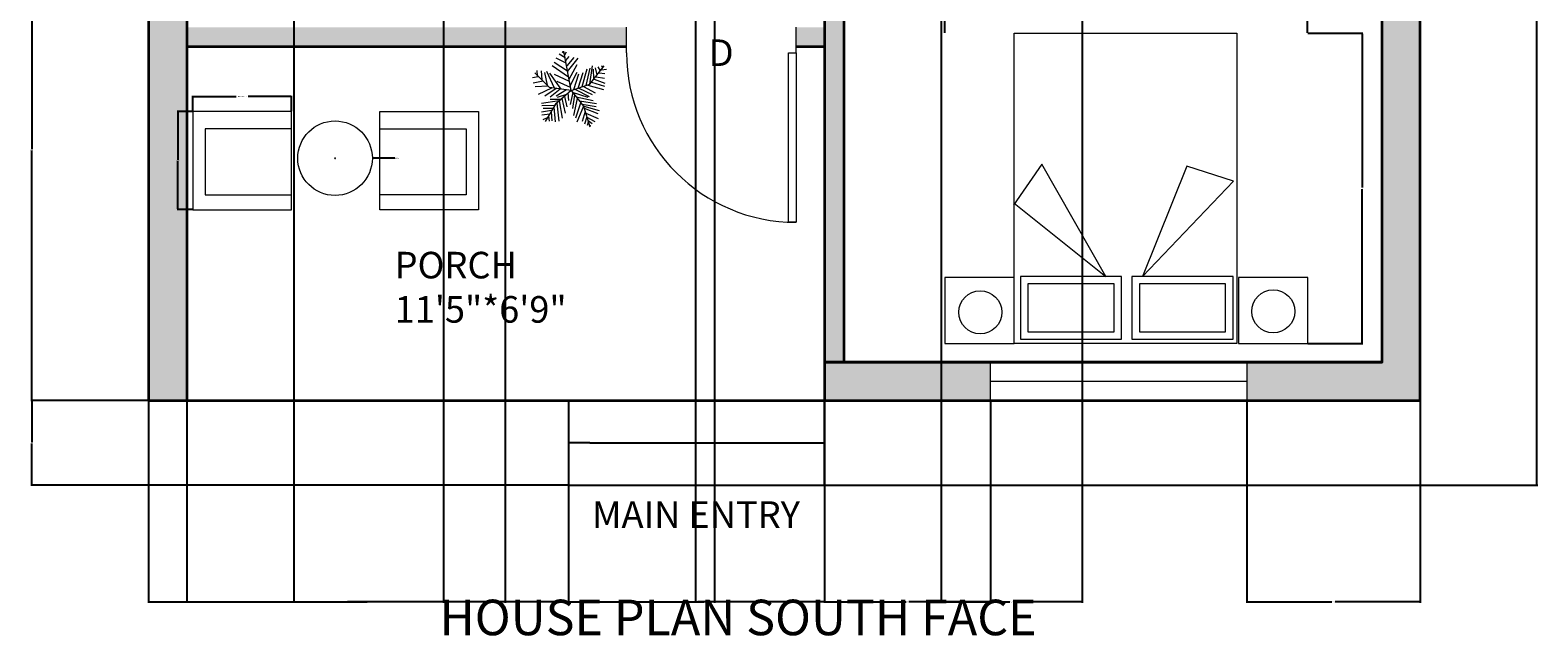
# Model space of a CAD drawing. Units: inches. Extents: x 1841 to 2210, y 2173 to 2736.
# Tile 1 of 4: x 1841 to 2197, y 2173 to 2316. Entities that reach past the tile are written whole.
import ezdxf

# ---------------------------------------------------------------- set-up
doc = ezdxf.new("R2010")
doc.units = ezdxf.units.IN
for name, color, linetype, lineweight in [('A-ANNO-DIMS', 2, 'Continuous', 18), ('A-AREA-IDEN', 10, 'Continuous', 18), ('A-FLOR-STRS', 7, 'Continuous', 25), ('A-FURN', 8, 'Continuous', 18), ('A-WALL', 7, 'Continuous', 35), ('A-WALL-PATT', 252, 'Continuous', 13), ('BED', 120, 'Continuous', 18), ('DOOR', 50, 'Continuous', 18), ('TEXT', 10, 'Continuous', 18), ('TREE', 70, 'Continuous', 13), ('WIN', 193, 'Continuous', 18)]:
    doc.layers.add(name, color=color, linetype=linetype, lineweight=lineweight)
doc.styles.get("Standard").update_dxf_attribs({"font": 'arial.ttf'})
doc.dimstyles.get("Standard").update_dxf_attribs({"dimtxt": 0.18, "dimasz": 0.18, "dimexe": 0.18, "dimexo": 0.0625, "dimgap": 0.09, "dimtad": 0, "dimtih": 1, "dimtoh": 1, "dimdec": 4, "dimzin": 0, "dimdsep": 46, "dimtxsty": 'Standard', "dimcen": 0.09, "dimadec": 0, "dimazin": 0, "dimtfac": 1, "dimtdec": 4, "dimtofl": 0, "dimtmove": 0, "dimatfit": 3, "dimfxl": 1, "dimtolj": 1, "dimtzin": 0, "dimarcsym": 0})

# ---------------------------------------------------------------- blocks, each defined once
blk = doc.blocks.new('*U2')
for p, q in [((0, 0), (0, -6)), ((40, 0), (40, -6))]:
    blk.add_line(p, q)
blk.add_lwpolyline([(0, 0), (0, 40), (1.75, 40), (1.75, 0)], close=True)
blk.add_arc((0, 0), 40, 0, 90)
blk = doc.blocks.new('*U6')
for p, q in [((-7.288, 39.707), (-21.778, 46.673)), ((-8.737, 47.138), (-17.069, 52.711)), ((-10.186, 53.64), (-13.084, 55.962)), ((0, 0), (-10.5, 57)), ((-9.099, 51.782), (-6.563, 55.962)), ((-7.65, 43.423), (-2.578, 49.46)), ((-5.839, 35.992), (4.667, 48.067)), ((-5.114, 27.632), (10.463, 46.673)), ((-31.5, 4.5), (-52.5, 25.5)), ((-48.585, 21.131), (-49.309, 29.026)), ((-43.513, 28.561), (-42.427, 15.558)), ((-38.442, 26.239), (-34.819, 7.663)), ((-35.544, 28.097), (-24.314, 3.947)), ((-14.533, 2.09), (-30.834, 25.31)), ((-3.665, 19.273), (-27.574, 35.527)), ((-5.114, 28.097), (-24.676, 40.636)), ((-24.314, 23.917), (-2.941, 13.7)), ((-2.941, 16.486), (8.652, 37.85)), ((-1.129, 6.734), (9.014, 26.704)), ((3.942, 1.625), (11.187, 24.381)), ((10.101, 3.483), (17.708, 26.239)), ((16.259, 5.805), (23.142, 31.348)), ((22.055, 7.198), (27.489, 32.277)), ((27, 9), (48, 36)), ((27.127, 9.056), (31.112, 35.992)), ((31.836, 30.883), (32.561, 16.486)), ((35.096, 32.741), (37.27, 22.524)), ((38.719, 34.134), (41.979, 28.561)), ((40.53, 25.775), (48.862, 24.846)), ((43.791, 29.954), (51.036, 30.883)), ((44.153, 36.456), (45.239, 32.741)), ((-47.498, 19.737), (-55.83, 18.344)), ((-40.615, 13.7), (-55.105, 10.913)), ((-33.37, 6.269), (-52.207, 5.34)), ((-28.299, 3.483), (-47.86, -5.805)), ((-21.416, 3.018), (-38.079, -8.128)), ((0, 0), (-31.5, 4.5)), ((-15.982, 2.09), (-30.11, -9.521)), ((0, 0), (-22.5, -19.5)), ((-6.563, 1.161), (-21.416, -8.128)), ((-20.691, 13.7), (-1.129, 4.876)), ((0, 0), (27, 9)), ((0, 0), (18, -22.5)), ((6.478, 1.625), (26.04, -8.592)), ((11.187, 3.483), (30.749, -5.805)), ((18.07, 5.805), (35.096, -3.483)), ((24.229, 7.663), (46.688, 1.625)), ((29.662, 12.307), (48.137, 6.269)), ((33.285, 16.486), (48.862, 10.913)), ((36.183, 19.737), (48.137, 17.88)), ((-17.431, -15.094), (-42.789, -18.809)), ((-24.314, -21.596), (-42.427, -22.06)), ((-22.5, -19.5), (-37.5, -45)), ((-15.257, -12.772), (-30.11, -12.772)), ((-20.691, -18.345), (-17.793, -44.352)), ((-6.563, -5.805), (-19.967, -9.985)), ((-17.069, -15.094), (-12.721, -40.172)), ((-13.446, -11.378), (-8.737, -32.741)), ((-9.461, -8.592), (-6.201, -23.453)), ((-4.752, -3.483), (-3.665, -14.629)), ((2.493, -3.019), (-1.491, -20.202)), ((1.769, -2.555), (24.229, -9.521)), ((5.029, -6.27), (2.131, -25.775)), ((9.014, -11.378), (3.58, -35.992)), ((14.085, -16.951), (6.478, -40.172)), ((7.565, -9.056), (32.198, -14.629)), ((12.274, -15.094), (36.907, -18.809)), ((16.259, -19.738), (36.183, -22.989)), ((-28.299, -29.026), (-42.789, -31.348)), ((-30.834, -34.135), (-42.427, -35.528)), ((-34.457, -39.708), (-40.978, -42.494)), ((-26.849, -26.24), (-40.253, -25.775)), ((-32.646, -36.921), (-31.921, -44.352)), ((-29.023, -30.884), (-27.936, -43.887)), ((-25.038, -23.918), (-22.865, -45.281)), ((18.07, -22.524), (8.289, -45.745)), ((20.244, -30.419), (15.897, -44.816)), ((18, -22.5), (27, -52.5)), ((18.433, -22.524), (40.53, -29.026)), ((19.157, -25.311), (38.719, -33.206)), ((22.78, -37.85), (19.519, -48.532)), ((21.331, -32.741), (39.081, -40.636)), ((22.78, -38.314), (34.372, -44.816)), ((24.591, -43.423), (30.749, -47.603)), ((24.591, -45.745), (23.142, -50.854)), ((26.764, -49.925), (28.213, -50.854))]:
    blk.add_line(p, q)
blk = doc.blocks.new('BED-DOUBLE-WITH-NIGHTSTANDS')
for p, q in [((33.07, 69.27), (15.79, 47.62)), ((42.3, 62.7), (32.63, 69.37)), ((15.79, 47.62), (42.3, 62.7)), ((15.79, 39), (38.26, 17.46)), ((41.84, 28.47), (15.79, 39)), ((38.26, 17.46), (41.84, 28.47))]:
    blk.add_line(p, q)
for points in [[(0, 69.27), (15.55, 69.27), (15.55, 85.57), (0, 85.57)], [(0, 69.27), (73.23, 69.27), (73.23, 16.72), (0, 16.72)], [(1.03, 43.89), (15.79, 43.89), (15.79, 67.76), (1.03, 67.76)], [(2.79, 45.65), (14.04, 45.65), (14.04, 66), (2.79, 66)], [(1.03, 17.59), (15.79, 17.59), (15.79, 41.47), (1.03, 41.47)], [(2.79, 19.35), (14.04, 19.35), (14.04, 39.71), (2.79, 39.71)], [(0, 0), (15.55, 0), (15.55, 16.3), (0, 16.3)]]:
    blk.add_lwpolyline(points, close=True)
for centre in [(7.36, 77.24), (7.58, 8.12)]:
    blk.add_circle(centre, 5.08)
blk = doc.blocks.new('WIN-60IN-NOM')
blk.add_line((4.5, 0), (4.5, 60.52))
blk.add_lwpolyline([(0, 60.52), (9, 60.52), (9, 0), (0, 0)], close=True)
blk = doc.blocks.new('CHAIR-PORCH')
for p, q in [((23.32, 23.17), (0, 23.17)), ((0, 23.17), (0, 0)), ((23.32, 19.05), (23.32, 23.17)), ((23.32, 0), (23.32, 11.27)), ((0, 0), (23.32, 0))]:
    blk.add_line(p, q)
blk.add_lwpolyline([(23.32, 19.05), (2.95, 19.05), (2.95, 3.5), (23.32, 3.5)], close=True)
blk = doc.blocks.new('*D16')
at = {"layer": 'A-ANNO-DIMS', "color": 0, "lineweight": -2, "transparency": 16777216}
for p, q in [((2056.93, 2315.11), (2056.93, 2328.07)), ((2057.11, 2327.89), (2098.62, 2327.89)), ((2142.32, 2327.89), (2100.81, 2327.89)), ((2142.5, 2315.11), (2142.5, 2328.07))]:
    blk.add_line(p, q, dxfattribs=at)
at = {"layer": 'A-ANNO-DIMS', "color": 0, "transparency": 16777216}
for points in [[(2057.11, 2327.92), (2057.11, 2327.86), (2056.93, 2327.89)], [(2142.32, 2327.92), (2142.32, 2327.86), (2142.5, 2327.89)]]:
    blk.add_solid(points, dxfattribs=at)
at = {"layer": 'Defpoints', "color": 0, "transparency": 16777216}
for p in [(2056.93, 2327.89), (2056.93, 2315.05), (2142.5, 2315.05)]:
    blk.add_point(p, dxfattribs=at)
at = {"layer": 'A-ANNO-DIMS', "color": 0, "transparency": 16777216, "insert": (2099.72, 2327.89), "char_height": 0.18, "attachment_point": 5}
blk.add_mtext('\\A1;BED SET 86 TYP.', dxfattribs=at)
blk = doc.blocks.new('*D17')
at = {"layer": 'A-ANNO-DIMS', "color": 0, "lineweight": -2, "transparency": 16777216}
for p, q in [((2142.57, 2315.05), (2155.52, 2315.05)), ((2155.34, 2314.87), (2155.34, 2278.62)), ((2155.34, 2242), (2155.34, 2278.25)), ((2142.57, 2241.82), (2155.52, 2241.82))]:
    blk.add_line(p, q, dxfattribs=at)
at = {"layer": 'A-ANNO-DIMS', "color": 0, "transparency": 16777216}
for points in [[(2155.31, 2314.87), (2155.37, 2314.87), (2155.34, 2315.05)], [(2155.31, 2242), (2155.37, 2242), (2155.34, 2241.82)]]:
    blk.add_solid(points, dxfattribs=at)
at = {"layer": 'Defpoints', "color": 0, "transparency": 16777216}
for p in [(2142.5, 2315.05), (2155.34, 2315.05), (2142.5, 2241.82)]:
    blk.add_point(p, dxfattribs=at)
at = {"layer": 'A-ANNO-DIMS', "color": 0, "transparency": 16777216, "insert": (2155.34, 2278.44), "char_height": 0.18, "attachment_point": 5}
blk.add_mtext('\\A1;73 TYP.', dxfattribs=at)
blk = doc.blocks.new('*D18')
at = {"layer": 'A-ANNO-DIMS', "color": 0, "lineweight": -2, "transparency": 16777216}
for p, q in [((1879.48, 2296.62), (1879.48, 2300.23)), ((1879.66, 2300.05), (1889.7, 2300.05)), ((1902.62, 2300.05), (1892.58, 2300.05)), ((1902.8, 2296.62), (1902.8, 2300.23))]:
    blk.add_line(p, q, dxfattribs=at)
at = {"layer": 'A-ANNO-DIMS', "color": 0, "transparency": 16777216}
for points in [[(1879.66, 2300.08), (1879.66, 2300.02), (1879.48, 2300.05)], [(1902.62, 2300.08), (1902.62, 2300.02), (1902.8, 2300.05)]]:
    blk.add_solid(points, dxfattribs=at)
at = {"layer": 'Defpoints', "color": 0, "transparency": 16777216}
for p in [(1902.8, 2300.05), (1879.48, 2296.55), (1902.8, 2296.55)]:
    blk.add_point(p, dxfattribs=at)
at = {"layer": 'A-ANNO-DIMS', "color": 0, "transparency": 16777216, "insert": (1891.14, 2300.05), "char_height": 0.18, "attachment_point": 5}
blk.add_mtext('\\A1;PORCH CHAIR 23 TYP.', dxfattribs=at)
blk = doc.blocks.new('*D19')
at = {"layer": 'A-ANNO-DIMS', "color": 0, "lineweight": -2, "transparency": 16777216}
for p, q in [((1879.42, 2296.55), (1875.8, 2296.55)), ((1875.98, 2296.37), (1875.98, 2285.15)), ((1875.98, 2273.57), (1875.98, 2284.79)), ((1879.42, 2273.39), (1875.8, 2273.39))]:
    blk.add_line(p, q, dxfattribs=at)
at = {"layer": 'A-ANNO-DIMS', "color": 0, "transparency": 16777216}
for points in [[(1875.95, 2296.37), (1876.01, 2296.37), (1875.98, 2296.55)], [(1875.95, 2273.57), (1876.01, 2273.57), (1875.98, 2273.39)]]:
    blk.add_solid(points, dxfattribs=at)
at = {"layer": 'Defpoints', "color": 0, "transparency": 16777216}
for p in [(1875.98, 2296.55), (1879.48, 2296.55), (1879.48, 2273.39)]:
    blk.add_point(p, dxfattribs=at)
at = {"layer": 'A-ANNO-DIMS', "color": 0, "transparency": 16777216, "insert": (1875.98, 2284.97), "char_height": 0.18, "attachment_point": 5}
blk.add_mtext('\\A1;23 TYP.', dxfattribs=at)
blk = doc.blocks.new('*D23')
at = {"layer": 'A-ANNO-DIMS', "color": 0, "lineweight": -2, "transparency": 16777216}
for p, q in [((2169.11, 2708.41), (2196.78, 2708.41)), ((2196.6, 2708.23), (2196.6, 2458.59)), ((2196.6, 2208.59), (2196.6, 2458.22)), ((2028.61, 2208.41), (2196.78, 2208.41))]:
    blk.add_line(p, q, dxfattribs=at)
at = {"layer": 'A-ANNO-DIMS', "color": 0, "transparency": 16777216}
for points in [[(2196.57, 2708.23), (2196.63, 2708.23), (2196.6, 2708.41)], [(2196.57, 2208.59), (2196.63, 2208.59), (2196.6, 2208.41)]]:
    blk.add_solid(points, dxfattribs=at)
at = {"layer": 'Defpoints', "color": 0, "transparency": 16777216}
for p in [(2169.05, 2708.41), (2196.6, 2708.41), (2028.55, 2208.41)]:
    blk.add_point(p, dxfattribs=at)
at = {"layer": 'A-ANNO-DIMS', "color": 0, "transparency": 16777216, "insert": (2196.6, 2458.41), "char_height": 0.18, "attachment_point": 5}
blk.add_mtext('\\A1;500', dxfattribs=at)
blk = doc.blocks.new('*D24')
at = {"layer": 'A-ANNO-DIMS', "color": 0, "lineweight": -2, "transparency": 16777216}
for p, q in [((1968.08, 2228.41), (1841.32, 2228.41)), ((1841.5, 2228.23), (1841.5, 2218.59)), ((1841.5, 2208.59), (1841.5, 2218.22)), ((1968.08, 2208.41), (1841.32, 2208.41))]:
    blk.add_line(p, q, dxfattribs=at)
at = {"layer": 'A-ANNO-DIMS', "color": 0, "transparency": 16777216}
for points in [[(1841.47, 2228.23), (1841.53, 2228.23), (1841.5, 2228.41)], [(1841.47, 2208.59), (1841.53, 2208.59), (1841.5, 2208.41)]]:
    blk.add_solid(points, dxfattribs=at)
at = {"layer": 'Defpoints', "color": 0, "transparency": 16777216}
for p in [(1841.5, 2228.41), (1968.15, 2228.41), (1968.15, 2208.41)]:
    blk.add_point(p, dxfattribs=at)
at = {"layer": 'A-ANNO-DIMS', "color": 0, "transparency": 16777216, "insert": (1841.5, 2218.41), "char_height": 0.18, "attachment_point": 5}
blk.add_mtext('\\A1;20', dxfattribs=at)
blk = doc.blocks.new('*D25')
at = {"layer": 'A-ANNO-DIMS', "color": 0, "lineweight": -2, "transparency": 16777216}
for p, q in [((1869.05, 2228.34), (1869.05, 2180.68)), ((1968.15, 2228.34), (1968.15, 2180.68)), ((1869.23, 2180.86), (1918.29, 2180.86)), ((1967.97, 2180.86), (1918.9, 2180.86))]:
    blk.add_line(p, q, dxfattribs=at)
at = {"layer": 'A-ANNO-DIMS', "color": 0, "transparency": 16777216}
for points in [[(1869.23, 2180.89), (1869.23, 2180.83), (1869.05, 2180.86)], [(1967.97, 2180.89), (1967.97, 2180.83), (1968.15, 2180.86)]]:
    blk.add_solid(points, dxfattribs=at)
at = {"layer": 'Defpoints', "color": 0, "transparency": 16777216}
for p in [(1869.05, 2228.41), (1968.15, 2228.41), (1968.15, 2180.86)]:
    blk.add_point(p, dxfattribs=at)
at = {"layer": 'A-ANNO-DIMS', "color": 0, "transparency": 16777216, "insert": (1918.6, 2180.86), "char_height": 0.18, "attachment_point": 5}
blk.add_mtext('\\A1;99.1', dxfattribs=at)
blk = doc.blocks.new('*D26')
at = {"layer": 'A-ANNO-DIMS', "color": 0, "lineweight": -2, "transparency": 16777216}
for p, q in [((1968.15, 2208.34), (1968.15, 2180.68)), ((2028.55, 2208.34), (2028.55, 2180.68)), ((1968.33, 2180.86), (1998.02, 2180.86)), ((2028.37, 2180.86), (1998.67, 2180.86))]:
    blk.add_line(p, q, dxfattribs=at)
at = {"layer": 'A-ANNO-DIMS', "color": 0, "transparency": 16777216}
for points in [[(1968.33, 2180.89), (1968.33, 2180.83), (1968.15, 2180.86)], [(2028.37, 2180.89), (2028.37, 2180.83), (2028.55, 2180.86)]]:
    blk.add_solid(points, dxfattribs=at)
at = {"layer": 'Defpoints', "color": 0, "transparency": 16777216}
for p in [(1968.15, 2208.41), (2028.55, 2208.41), (2028.55, 2180.86)]:
    blk.add_point(p, dxfattribs=at)
at = {"layer": 'A-ANNO-DIMS', "color": 0, "transparency": 16777216, "insert": (1998.35, 2180.86), "char_height": 0.18, "attachment_point": 5}
blk.add_mtext('\\A1;60.4', dxfattribs=at)
blk = doc.blocks.new('*D27')
at = {"layer": 'A-ANNO-DIMS', "color": 0, "lineweight": -2, "transparency": 16777216}
for p, q in [((2028.55, 2228.34), (2028.55, 2180.68)), ((2067.65, 2228.34), (2067.65, 2180.68)), ((2028.73, 2180.86), (2047.8, 2180.86)), ((2067.47, 2180.86), (2048.41, 2180.86))]:
    blk.add_line(p, q, dxfattribs=at)
at = {"layer": 'A-ANNO-DIMS', "color": 0, "transparency": 16777216}
for points in [[(2028.73, 2180.89), (2028.73, 2180.83), (2028.55, 2180.86)], [(2067.47, 2180.89), (2067.47, 2180.83), (2067.65, 2180.86)]]:
    blk.add_solid(points, dxfattribs=at)
at = {"layer": 'Defpoints', "color": 0, "transparency": 16777216}
for p in [(2028.55, 2228.41), (2067.65, 2228.41), (2067.65, 2180.86)]:
    blk.add_point(p, dxfattribs=at)
at = {"layer": 'A-ANNO-DIMS', "color": 0, "transparency": 16777216, "insert": (2048.1, 2180.86), "char_height": 0.18, "attachment_point": 5}
blk.add_mtext('\\A1;39.1', dxfattribs=at)
blk = doc.blocks.new('*D28')
at = {"layer": 'A-ANNO-DIMS', "color": 0, "lineweight": -2, "transparency": 16777216}
for p, q in [((2128.17, 2228.34), (2128.17, 2180.68)), ((2169.05, 2228.34), (2169.05, 2180.68)), ((2128.35, 2180.86), (2148.21, 2180.86)), ((2168.87, 2180.86), (2149.01, 2180.86))]:
    blk.add_line(p, q, dxfattribs=at)
at = {"layer": 'A-ANNO-DIMS', "color": 0, "transparency": 16777216}
for points in [[(2128.35, 2180.89), (2128.35, 2180.83), (2128.17, 2180.86)], [(2168.87, 2180.89), (2168.87, 2180.83), (2169.05, 2180.86)]]:
    blk.add_solid(points, dxfattribs=at)
at = {"layer": 'Defpoints', "color": 0, "transparency": 16777216}
for p in [(2128.17, 2228.41), (2169.05, 2228.41), (2128.17, 2180.86)]:
    blk.add_point(p, dxfattribs=at)
at = {"layer": 'A-ANNO-DIMS', "color": 0, "transparency": 16777216, "insert": (2148.61, 2180.86), "char_height": 0.18, "attachment_point": 5}
blk.add_mtext('\\A1;40.88', dxfattribs=at)
blk = doc.blocks.new('*D29')
at = {"layer": 'A-ANNO-DIMS', "color": 0, "lineweight": -2, "transparency": 16777216}
for p, q in [((1868.99, 2346.57), (1841.32, 2346.57)), ((1841.5, 2346.39), (1841.5, 2287.67)), ((1841.5, 2228.59), (1841.5, 2287.31)), ((1868.99, 2228.41), (1841.32, 2228.41))]:
    blk.add_line(p, q, dxfattribs=at)
at = {"layer": 'A-ANNO-DIMS', "color": 0, "transparency": 16777216}
for points in [[(1841.47, 2346.39), (1841.53, 2346.39), (1841.5, 2346.57)], [(1841.47, 2228.59), (1841.53, 2228.59), (1841.5, 2228.41)]]:
    blk.add_solid(points, dxfattribs=at)
at = {"layer": 'Defpoints', "color": 0, "transparency": 16777216}
for p in [(1841.5, 2346.57), (1869.05, 2346.57), (1869.05, 2228.41)]:
    blk.add_point(p, dxfattribs=at)
at = {"layer": 'A-ANNO-DIMS', "color": 0, "transparency": 16777216, "insert": (1841.5, 2287.49), "char_height": 0.18, "attachment_point": 5}
blk.add_mtext('\\A1;118.17', dxfattribs=at)
blk = doc.blocks.new('*D40')
at = {"layer": 'A-ANNO-DIMS', "color": 0, "lineweight": -2, "transparency": 16777216}
for p, q in [((1903.36, 2465.22), (1903.36, 2180.68)), ((1938.67, 2465.22), (1938.67, 2180.68)), ((1903.54, 2180.86), (1920.64, 2180.86)), ((1938.49, 2180.86), (1921.39, 2180.86))]:
    blk.add_line(p, q, dxfattribs=at)
at = {"layer": 'A-ANNO-DIMS', "color": 0, "transparency": 16777216}
for points in [[(1903.54, 2180.89), (1903.54, 2180.83), (1903.36, 2180.86)], [(1938.49, 2180.89), (1938.49, 2180.83), (1938.67, 2180.86)]]:
    blk.add_solid(points, dxfattribs=at)
at = {"layer": 'Defpoints', "color": 0, "transparency": 16777216}
for p in [(1903.36, 2465.28), (1938.67, 2465.28), (1938.67, 2180.86)]:
    blk.add_point(p, dxfattribs=at)
at = {"layer": 'A-ANNO-DIMS', "color": 0, "transparency": 16777216, "insert": (1921.01, 2180.86), "char_height": 0.18, "attachment_point": 5}
blk.add_mtext('\\A1;35.31', dxfattribs=at)
blk = doc.blocks.new('*D42')
at = {"layer": 'A-ANNO-DIMS', "color": 0, "lineweight": -2, "transparency": 16777216}
for p, q in [((1878.05, 2550.84), (1878.05, 2180.68)), ((1953.17, 2550.84), (1953.17, 2180.68)), ((1878.23, 2180.86), (1915.22, 2180.86)), ((1952.99, 2180.86), (1916, 2180.86))]:
    blk.add_line(p, q, dxfattribs=at)
at = {"layer": 'A-ANNO-DIMS', "color": 0, "transparency": 16777216}
for points in [[(1878.23, 2180.89), (1878.23, 2180.83), (1878.05, 2180.86)], [(1952.99, 2180.89), (1952.99, 2180.83), (1953.17, 2180.86)]]:
    blk.add_solid(points, dxfattribs=at)
at = {"layer": 'Defpoints', "color": 0, "transparency": 16777216}
for p in [(1878.05, 2550.91), (1953.17, 2550.91), (1953.17, 2180.86)]:
    blk.add_point(p, dxfattribs=at)
at = {"layer": 'A-ANNO-DIMS', "color": 0, "transparency": 16777216, "insert": (1915.61, 2180.86), "char_height": 0.18, "attachment_point": 5}
blk.add_mtext('\\A1;75.12', dxfattribs=at)
blk = doc.blocks.new('*D43')
at = {"layer": 'A-ANNO-DIMS', "color": 0, "lineweight": -2, "transparency": 16777216}
for p, q in [((2056.06, 2637.84), (2056.06, 2180.68)), ((2089.3, 2637.84), (2089.3, 2180.68)), ((2056.24, 2180.86), (2072.22, 2180.86)), ((2089.12, 2180.86), (2073.14, 2180.86))]:
    blk.add_line(p, q, dxfattribs=at)
at = {"layer": 'A-ANNO-DIMS', "color": 0, "transparency": 16777216}
for points in [[(2056.24, 2180.89), (2056.24, 2180.83), (2056.06, 2180.86)], [(2089.12, 2180.89), (2089.12, 2180.83), (2089.3, 2180.86)]]:
    blk.add_solid(points, dxfattribs=at)
at = {"layer": 'Defpoints', "color": 0, "transparency": 16777216}
for p in [(2056.06, 2637.91), (2089.3, 2637.91), (2089.3, 2180.86)]:
    blk.add_point(p, dxfattribs=at)
at = {"layer": 'A-ANNO-DIMS', "color": 0, "transparency": 16777216, "insert": (2072.68, 2180.86), "char_height": 0.18, "attachment_point": 5}
blk.add_mtext('\\A1;33.234', dxfattribs=at)
blk = doc.blocks.new('*D45')
at = {"layer": 'A-ANNO-DIMS', "color": 0, "lineweight": -2, "transparency": 16777216}
for p, q in [((1998.05, 2540.69), (1998.05, 2180.68)), ((2002.55, 2540.69), (2002.55, 2180.68)), ((1998.23, 2180.86), (2000.04, 2180.86)), ((2002.37, 2180.86), (2000.56, 2180.86))]:
    blk.add_line(p, q, dxfattribs=at)
at = {"layer": 'A-ANNO-DIMS', "color": 0, "transparency": 16777216}
for points in [[(1998.23, 2180.89), (1998.23, 2180.83), (1998.05, 2180.86)], [(2002.37, 2180.89), (2002.37, 2180.83), (2002.55, 2180.86)]]:
    blk.add_solid(points, dxfattribs=at)
at = {"layer": 'Defpoints', "color": 0, "transparency": 16777216}
for p in [(1998.05, 2540.75), (2002.55, 2540.75), (2002.55, 2180.86)]:
    blk.add_point(p, dxfattribs=at)
at = {"layer": 'A-ANNO-DIMS', "color": 0, "transparency": 16777216, "insert": (2000.3, 2180.86), "char_height": 0.18, "attachment_point": 5}
blk.add_mtext('\\A1;4.5', dxfattribs=at)
blk = doc.blocks.new('*D51')
at = {"layer": 'A-ANNO-DIMS', "color": 0, "lineweight": -2, "transparency": 16777216}
for p, q in [((1912.97, 2285.53), (1913.15, 2285.53)), ((1913.06, 2285.44), (1913.06, 2285.62)), ((1927.13, 2285.53), (1922.03, 2285.53))]:
    blk.add_line(p, q, dxfattribs=at)
at = {"layer": 'A-ANNO-DIMS', "color": 0, "transparency": 16777216}
blk.add_solid([(1922.03, 2285.56), (1922.03, 2285.5), (1921.85, 2285.53)], dxfattribs=at)
at = {"layer": 'Defpoints', "color": 0, "transparency": 16777216}
for p in [(1904.26, 2285.53), (1921.85, 2285.53)]:
    blk.add_point(p, dxfattribs=at)
at = {"layer": 'A-ANNO-DIMS', "color": 0, "transparency": 16777216, "insert": (1927.62, 2285.53), "char_height": 0.18, "attachment_point": 5}
blk.add_mtext('\\A1;∅17.59', dxfattribs=at)

msp = doc.modelspace()

# ---------------------------------------------------------------- hatches: boundary and pattern name
at = {"layer": 'A-WALL-PATT'}
h = msp.add_hatch(color=256, dxfattribs=at)
h.dxf.hatch_style = 1
h.paths.add_polyline_path([(2169.0509, 2546.8192), (2160.3559, 2546.8192), (2160.3559, 2545.451), (2160.3559, 2529.1476), (2160.0509, 2237.4052), (2128.1686, 2237.4052), (2128.1686, 2228.4052), (2169.0509, 2228.4052)])
h.paths.add_polyline_path([(2067.6527, 2237.4052), (2028.5509, 2237.4052), (2028.5509, 2228.4052), (2067.6527, 2228.4052)])
h.paths.add_polyline_path([(2033.0509, 2321.9228), (2028.5509, 2321.9228), (2028.5509, 2237.4052), (2033.0509, 2237.4052)])
h.paths.add_polyline_path([(2160.0509, 2369.9052), (2052.0509, 2369.9052), (2052.0509, 2380.7227), (2047.5509, 2380.7227), (2047.5509, 2369.9052), (2028.5509, 2369.9052), (2028.5509, 2364.1588), (2028.5509, 2361.9228), (2033.0509, 2361.9228), (2033.0509, 2365.4052), (2050.3181, 2365.4052), (2160.0509, 2365.4052)])
h.paths.add_polyline_path([(1878.0509, 2346.5722), (1869.0509, 2346.5722), (1869.0509, 2228.4052), (1878.0509, 2228.4052), (1878.0509, 2237.4052)])
h.paths.add_polyline_path([(1981.8009, 2316.4052), (1878.0509, 2316.4052), (1878.0509, 2311.9052), (1981.8009, 2311.9052)])
h.paths.add_polyline_path([(1978.2584, 2442.9052), (1878.0509, 2442.9052), (1878.0509, 2438.4052), (1914.0509, 2438.4052), (1978.2584, 2438.4052)])
h.paths.add_polyline_path([(1878.0509, 2468.4052), (1869.0509, 2468.4052), (1869.0509, 2407.0881), (1878.0509, 2407.0881), (1878.0509, 2438.4052)])
h.paths.add_polyline_path([(2028.5509, 2442.9052), (2018.2584, 2442.9052), (2018.2584, 2438.4052), (2028.5509, 2438.4052)])
h.paths.add_polyline_path([(2131.5968, 2498.9052), (2002.5509, 2498.9052), (2002.5509, 2500.7487), (1998.0509, 2500.7487), (1998.0509, 2494.4052), (2131.5968, 2494.4052)])
h.paths.add_polyline_path([(2033.0509, 2489.9052), (2033.0509, 2494.4052), (2028.5509, 2494.4052), (2028.5509, 2489.9052), (2028.5509, 2417.9052), (2131.5509, 2417.9052), (2131.5509, 2422.4052), (2033.0509, 2422.4052), (2033.0294, 2446.4052)])
h.paths.add_polyline_path([(1953.1667, 2555.4052), (1878.0509, 2555.4052), (1878.0509, 2550.9052), (1953.1667, 2550.9052)], flags=17)
h.paths.add_polyline_path([(1878.0509, 2699.4052), (2160.0509, 2699.4052), (2160.0509, 2607.3351), (2169.0509, 2607.3351), (2169.0509, 2708.4052), (1869.0509, 2708.4052), (1869.0509, 2528.9211), (1878.0509, 2528.9211), (1878.0509, 2550.9052), (1878.0509, 2555.4052)])
h.paths.add_polyline_path([(1998.0509, 2555.4052), (1993.1667, 2555.4052), (1993.1667, 2550.9052), (1998.0509, 2550.9052)], flags=17)
h.paths.add_polyline_path([(2002.5509, 2550.9052), (1998.0509, 2550.9052), (1998.0509, 2540.7487), (2002.5509, 2540.7487)], flags=17)
h.paths.add_polyline_path([(2002.5509, 2576.8157), (2002.5509, 2607.2805), (2002.5509, 2699.4052), (1998.0509, 2699.4052), (1998.0509, 2555.4052), (1998.0509, 2550.9052), (2002.5509, 2550.9052)], flags=17)
h.paths.add_polyline_path([(2160.0509, 2642.4052), (2089.2965, 2642.4052), (2089.2965, 2637.9052), (2160.0509, 2637.9052)], flags=17)
h.paths.add_polyline_path([(2056.0629, 2642.4052), (2054.0509, 2642.4052), (2054.0509, 2699.4052), (2049.5509, 2699.4052), (2049.5509, 2642.4052), (2002.5509, 2642.4052), (2002.5509, 2637.9052), (2054.0509, 2637.9052), (2056.0629, 2637.9052)], flags=17)
h.paths.add_polyline_path([(1924.594, 2243.1802), (1965.0263, 2243.1802), (1965.0263, 2266.5581), (1924.594, 2266.5581)], flags=9)
h.paths.add_polyline_path([(2082.2056, 2327.2752), (2130.8731, 2327.2752), (2130.8731, 2350.6531), (2082.2056, 2350.6531)], flags=9)
h.paths.add_polyline_path([(2000.1077, 2344.9343), (2000.1077, 2400.666), (1976.7298, 2400.666), (1976.7298, 2344.9343)], flags=9)
h.paths.add_polyline_path([(2161.6353, 2440.9897), (2161.6353, 2476.9732), (2138.2574, 2476.9732), (2138.2574, 2440.9897)], flags=24)
h.paths.add_polyline_path([(2044.2273, 2462.409), (2085.775, 2462.409), (2085.775, 2485.7869), (2044.2273, 2485.7869)], flags=25)
h.paths.add_polyline_path([(1940.3738, 2512.1813), (2005.58, 2512.1813), (2005.58, 2535.5592), (1940.3738, 2535.5592)], flags=9)
h.paths.add_polyline_path([(2088.5551, 2604.7497), (2142.0901, 2604.7497), (2142.0901, 2628.1276), (2088.5551, 2628.1276)], flags=25)
h.paths.add_polyline_path([(2110.3045, 2670.6273), (2145.8692, 2670.6273), (2145.8692, 2694.0052), (2110.3045, 2694.0052)], flags=25)
h.paths.add_polyline_path([(2002.7596, 2670.6273), (2043.2176, 2670.6273), (2043.2176, 2694.0052), (2002.7596, 2694.0052)], flags=24)
h.paths.add_polyline_path([(1907.1501, 2670.6273), (1955.8175, 2670.6273), (1955.8175, 2694.0052), (1907.1501, 2694.0052)], flags=25)
h = msp.add_hatch(color=256, dxfattribs=at)
h.dxf.hatch_style = 1
h.paths.add_polyline_path([(2028.5509, 2316.4052), (2021.8009, 2316.4052), (2021.8009, 2311.9052), (2028.5509, 2311.9052)])
h.paths.add_polyline_path([(2052.0509, 2417.9052), (2047.5509, 2417.9052), (2047.5509, 2414.752), (2052.0509, 2414.752)])

# ---------------------------------------------------------------- linework, layer by layer
at = {"layer": 'A-FLOR-STRS'}
for p, q in [((1968.1458, 2228.4052), (1968.1458, 2218.4052)), ((2028.5509, 2218.4052), (2028.5509, 2230.0845)), ((2028.5509, 2208.4052), (2028.5509, 2224.2449)), ((1968.1458, 2218.4052), (1968.1458, 2208.4052)), ((1973.1458, 2218.4052), (1968.1458, 2218.4052)), ((1973.1458, 2218.4052), (2028.5509, 2218.4052)), ((1968.1458, 2208.4052), (2028.5509, 2208.4052))]:
    msp.add_line(p, q, dxfattribs=at)
at = {"layer": 'A-FURN'}
msp.add_circle((1913.0556, 2285.5281), 8.7955, dxfattribs=at)
at = {"layer": 'A-WALL'}
for p, q in [((2028.5509, 2321.9228), (2028.5509, 2237.4052)), ((2033.0509, 2321.9228), (2033.0509, 2237.4052)), ((1878.0509, 2311.9052), (1981.8009, 2311.9052)), ((2021.8009, 2311.9052), (2028.5509, 2311.9052)), ((1878.0509, 2237.4052), (1878.0509, 2228.4052)), ((2160.0509, 2237.4052), (2028.5509, 2237.4052)), ((2028.5509, 2237.4052), (2028.5509, 2228.4052))]:
    msp.add_line(p, q, dxfattribs=at)
msp.add_lwpolyline([(1869.0509, 2228.4052), (2169.0509, 2228.4052), (2169.0509, 2708.4052), (1869.0509, 2708.4052)], close=True, dxfattribs=at)
msp.add_lwpolyline([(2028.5509, 2237.4052), (2160.0509, 2237.4052), (2160.0509, 2699.4052), (1878.0509, 2699.4052), (1878.0509, 2237.4052)], dxfattribs=at)

# ---------------------------------------------------------------- block references
at = {"layer": 'A-FURN'}
msp.add_blockref('CHAIR-PORCH', (1879.481, 2273.388), dxfattribs=at)
at = {"layer": 'A-FURN', "extrusion": (0, 0, -1), "zscale": -1}
msp.add_blockref('CHAIR-PORCH', (-1946.9286, 2273.388), dxfattribs=at)
at = {"layer": 'BED', "rotation": 90.00000000000104}
msp.add_blockref('BED-DOUBLE-WITH-NIGHTSTANDS', (2142.5045, 2241.8221), dxfattribs=at)
at = {"layer": 'DOOR', "rotation": 180}
msp.add_blockref('*U2', (2021.8009, 2310.4052), dxfattribs=at)
at = {"layer": 'TREE', "xscale": 0.1629161344806782, "yscale": 0.1629161344806782, "zscale": 0.1629161344806782}
msp.add_blockref('*U6', (1968.7395, 2301.4867), dxfattribs=at)
at = {"layer": 'WIN', "rotation": 270.0000000000007}
msp.add_blockref('WIN-60IN-NOM', (2067.6525, 2237.4051), dxfattribs=at)

# ---------------------------------------------------------------- texts
at = {"layer": 'A-AREA-IDEN', "insert": (1927.1133, 2263.4448), "char_height": 6.26506, "attachment_point": 1}
msp.add_mtext_dynamic_manual_height_columns('PORCH\\P11\'5"*6\'9"', width=112.651532, gutter_width=31.3253, heights=[0], dxfattribs=at)
at = {"layer": 'TEXT', "attachment_point": 1}
for s, width, gutter_width, insert, char_height in [('D', 112.651532, 31.3253, (2001.2055, 2313.544), 6.2651), ('MAIN ENTRY', 112.651532, 31.3253, (1973.6962, 2204.6111), 6.26506), ('HOUSE PLAN SOUTH FACE', 871.627973, 41.8832, (1937.6918, 2181.3999), 8.376642)]:
    msp.add_mtext_dynamic_manual_height_columns(s, width=width, gutter_width=gutter_width, heights=[0], dxfattribs=dict(at, insert=insert, char_height=char_height))

# ---------------------------------------------------------------- dimensions: what is measured, and where the dimension line sits
at = {"layer": 'A-ANNO-DIMS'}
for base, p1, p2, override, picture, middle in [((2196.6009, 2708.4052), (2028.5509, 2208.4052), (2169.0509, 2708.4052), {"dimdec": 0, "dimlfac": 1, "dimrnd": 0, "dimzin": 0, "dimdsep": 46, "dimlunit": 2}, '*D23', (2196.6009, 2458.4052)), ((1841.5009, 2346.5722), (1869.0509, 2228.4052), (1869.0509, 2346.5722), {"dimdec": 2, "dimlfac": 1, "dimrnd": 0, "dimzin": 0, "dimdsep": 46, "dimlunit": 2}, '*D29', (1841.5009, 2287.4887)), ((1841.5009, 2228.4052), (1968.1458, 2208.4052), (1968.1458, 2228.4052), {"dimdec": 0, "dimlfac": 1, "dimrnd": 0, "dimzin": 0, "dimdsep": 46, "dimlunit": 2}, '*D24', (1841.5009, 2218.4052))]:
    dim = msp.add_linear_dim(base=base, p1=p1, p2=p2, angle=90, dimstyle='Standard', override=override, dxfattribs=at)
    dim.commit()
    dim.dimension.update_dxf_attribs({"geometry": picture, "text_midpoint": middle})
for base, p1, p2, override, picture, middle in [((2089.2965, 2180.8552), (2056.0629, 2637.9052), (2089.2965, 2637.9052), {"dimdec": 3, "dimlfac": 1, "dimrnd": 0, "dimzin": 0, "dimdsep": 46, "dimlunit": 2}, '*D43', (2072.6797, 2180.8552)), ((1953.1667, 2180.8552), (1878.0509, 2550.9052), (1953.1667, 2550.9052), {"dimdec": 2, "dimlfac": 1, "dimrnd": 0, "dimzin": 0, "dimdsep": 46, "dimlunit": 2}, '*D42', (1915.6088, 2180.8552)), ((2002.5509, 2180.8552), (1998.0509, 2540.7487), (2002.5509, 2540.7487), {"dimdec": 1, "dimlfac": 1, "dimrnd": 0, "dimzin": 0, "dimdsep": 46, "dimlunit": 2}, '*D45', (2000.3009, 2180.8552)), ((1938.6659, 2180.8552), (1903.3594, 2465.2791), (1938.6659, 2465.2791), {"dimdec": 2, "dimlfac": 1, "dimrnd": 0, "dimzin": 0, "dimdsep": 46, "dimlunit": 2}, '*D40', (1921.0127, 2180.8552)), ((1968.1458, 2180.8552), (1869.0509, 2228.4052), (1968.1458, 2228.4052), {"dimdec": 1, "dimlfac": 1, "dimrnd": 0, "dimzin": 0, "dimdsep": 46, "dimlunit": 2}, '*D25', (1918.5983, 2180.8552)), ((2067.6527, 2180.8552), (2028.5509, 2228.4052), (2067.6527, 2228.4052), {"dimdec": 1, "dimlfac": 1, "dimrnd": 0, "dimzin": 0, "dimdsep": 46, "dimlunit": 2}, '*D27', (2048.1018, 2180.8552)), ((2128.1686, 2180.8552), (2169.0509, 2228.4052), (2128.1686, 2228.4052), {"dimdec": 2, "dimlfac": 1, "dimrnd": 0, "dimzin": 0, "dimdsep": 46, "dimlunit": 2}, '*D28', (2148.6098, 2180.8552)), ((2028.5509, 2180.8552), (1968.1458, 2208.4052), (2028.5509, 2208.4052), {"dimdec": 1, "dimlfac": 1, "dimrnd": 0, "dimzin": 0, "dimdsep": 46, "dimlunit": 2}, '*D26', (1998.3483, 2180.8552))]:
    dim = msp.add_linear_dim(base=base, p1=p1, p2=p2, dimstyle='Standard', override=override, dxfattribs=at)
    dim.commit()
    dim.dimension.update_dxf_attribs({"geometry": picture, "text_midpoint": middle})
for base, p1, p2, angle, text, picture, middle in [((2056.93, 2327.8857), (2142.505, 2315.0494), (2056.93, 2315.0494), 180, 'BED SET <> TYP.', '*D16', (2099.7175, 2327.8857)), ((2155.3413, 2315.0494), (2142.505, 2241.822), (2142.505, 2315.0494), 90, '<> TYP.', '*D17', (2155.3413, 2278.4357)), ((1875.9829, 2296.5549), (1879.4813, 2273.3885), (1879.4813, 2296.5549), 90, '<> TYP.', '*D19', (1875.9829, 2284.9717))]:
    dim = msp.add_linear_dim(base=base, p1=p1, p2=p2, angle=angle, text=text, dimstyle='Standard', override={"dimdec": 0, "dimlfac": 1, "dimrnd": 0, "dimzin": 0, "dimdsep": 46, "dimlunit": 2}, dxfattribs=at)
    dim.commit()
    dim.dimension.update_dxf_attribs({"geometry": picture, "text_midpoint": middle})
dim = msp.add_linear_dim(base=(1902.8037, 2300.0533), p1=(1879.4813, 2296.5549), p2=(1902.8037, 2296.5549), text='PORCH CHAIR <> TYP.', dimstyle='Standard', override={"dimdec": 0, "dimlfac": 1, "dimrnd": 0, "dimzin": 0, "dimdsep": 46, "dimlunit": 2}, dxfattribs=at)
dim.commit()
dim.dimension.update_dxf_attribs({"geometry": '*D18', "text_midpoint": (1891.1425, 2300.0533)})
dim = msp.add_diameter_dim_2p(p1=(1904.2601, 2285.5281), p2=(1921.8511, 2285.528), dimstyle='Standard', override={"dimdec": 2, "dimlfac": 1, "dimrnd": 0, "dimzin": 0, "dimdsep": 46, "dimlunit": 2}, dxfattribs=at)
dim.commit()
dim.dimension.update_dxf_attribs({"geometry": '*D51', "text_midpoint": (1927.1284, 2285.528), "dimtype": 163})

doc.saveas('drawing.dxf')
